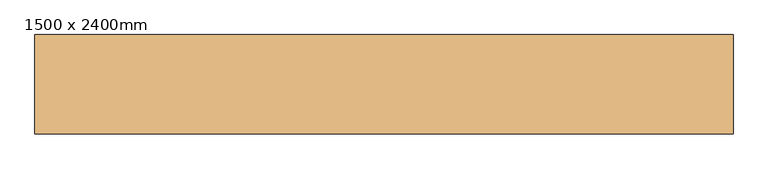
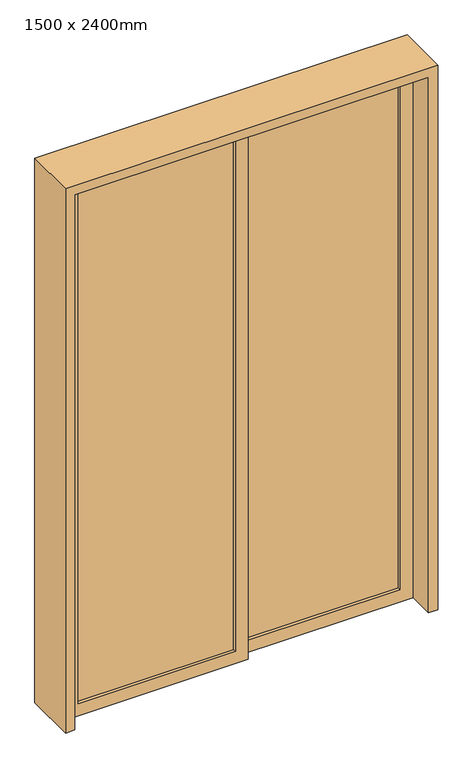
"""IFC4 building model written with IfcOpenShell, lengths in millimetres: door geometry, 1500 x 2400mm."""

from ifc_helpers import new_model, si_unit, frame, origin, place, context, project, spatial, polyline, outline, extrude, source, transform, mapped, element, save


def door_1500_x_2400mm_f3db478b(model_context):
    return source(origin(), model_context, "Body", "SweptSolid", [
        extrude(outline(polyline([(780.7580012, 26.6666667), (780.7580012, 13.3333333), (113.2580012, 13.3333333), (113.2580012, 26.6666667), (780.7580012, 26.6666667)])), frame((0.0, 0.0, 55.0), z_axis=(0.0, 0.0, 1.0), x_axis=(1.0, 0.0, 0.0)), (0.0, 0.0, 1.0), 2290.0),
        extrude(outline(polyline([(0.0, 835.7580012), (2400.0, 835.7580012), (2400.0, 58.2580012), (0.0, 58.2580012), (0.0, 835.7580012)]), holes=[polyline([(55.0, 780.7580012), (55.0, 113.2580012), (2345.0, 113.2580012), (2345.0, 780.7580012), (55.0, 780.7580012)])]), frame((0.0, 0.0, 0.0), z_axis=(0.0, 1.0, 0.0), x_axis=(0.0, 0.0, 1.0)), (0.0, 0.0, 1.0), 40.0),
        extrude(outline(polyline([(58.2580012, -13.3333333), (58.2580012, -26.6666667), (-609.2419988, -26.6666667), (-609.2419988, -13.3333333), (58.2580012, -13.3333333)])), frame((0.0, 0.0, 55.0), z_axis=(0.0, 0.0, 1.0), x_axis=(1.0, 0.0, 0.0)), (0.0, 0.0, 1.0), 2290.0),
        extrude(outline(polyline([(0.0, 113.2580012), (2400.0, 113.2580012), (2400.0, -664.2419988), (0.0, -664.2419988), (0.0, 113.2580012)]), holes=[polyline([(55.0, 58.2580012), (55.0, -609.2419988), (2345.0, -609.2419988), (2345.0, 58.2580012), (55.0, 58.2580012)])]), frame((0.0, -40.0, 0.0), z_axis=(0.0, 1.0, 0.0), x_axis=(0.0, 0.0, 1.0)), (0.0, 0.0, 1.0), 40.0),
        extrude(outline(polyline([(0.0, -704.2419988), (0.0, -664.2419988), (2400.0, -664.2419988), (2400.0, 835.7580012), (0.0, 835.7580012), (0.0, 875.7580012), (2440.0, 875.7580012), (2440.0, -704.2419988), (0.0, -704.2419988)])), frame((0.0, -112.5, 0.0), z_axis=(0.0, 1.0, 0.0), x_axis=(0.0, 0.0, 1.0)), (0.0, 0.0, 1.0), 225.0),
    ])


if __name__ == "__main__":
    model = new_model("IFC4")
    model_context = context("Model", 3, world=origin())
    ifc_project = project(units=[si_unit("LENGTHUNIT", "METRE", prefix="MILLI")], contexts=[model_context])
    site = spatial("IfcSite", under=ifc_project)
    building = spatial("IfcBuilding", under=site)
    placement = place(None, origin())
    door_1500_x_2400mm_shape = door_1500_x_2400mm_f3db478b(model_context)
    element("IfcDoor", 1, ObjectType="1500 x 2400mm", at=placement, inside=building, context=model_context, shape_type="MappedRepresentation", body=[
        mapped(door_1500_x_2400mm_shape, transform((0.0, 0.0, 0.0), x_axis=(1.0, 0.0, 0.0), y_axis=(0.0, 1.0, 0.0), z_axis=(0.0, 0.0, 1.0))),
    ])
    save(model, "model.ifc")

# Revit data of these elements
# Type "1500 x 2400mm"
#   Type Mark = "47"
#   Operation = "UserDefined"
#   Analytic Construction = "<None>"
#   Width = 1500 mm
#   Thickness = 40 mm
#   Rough Width = 1580 mm
#   Rough Height = 2440 mm
#   Panel Width = 777.5 mm
#   Panel Frame = 55 mm
#   Height = 2400 mm
#   Frame Depth = 40 mm
#   Define Thermal Properties by = 1
#   Glass Material = Sliding Door Glass
#   Frame Material = Sliding Door Frame
#   Function = (empty or 0)
# Element 1 (IfcDoor, "1500 x 2400mm")
#   Materials on its faces: "Sliding Door Frame", "Sliding Door Glass"
# Materials
#   "Sliding Door Glass": colour RGB 247 247 247, transparency 0.68
#   "Sliding Door Frame": colour RGB 160 107 8, transparency 0
